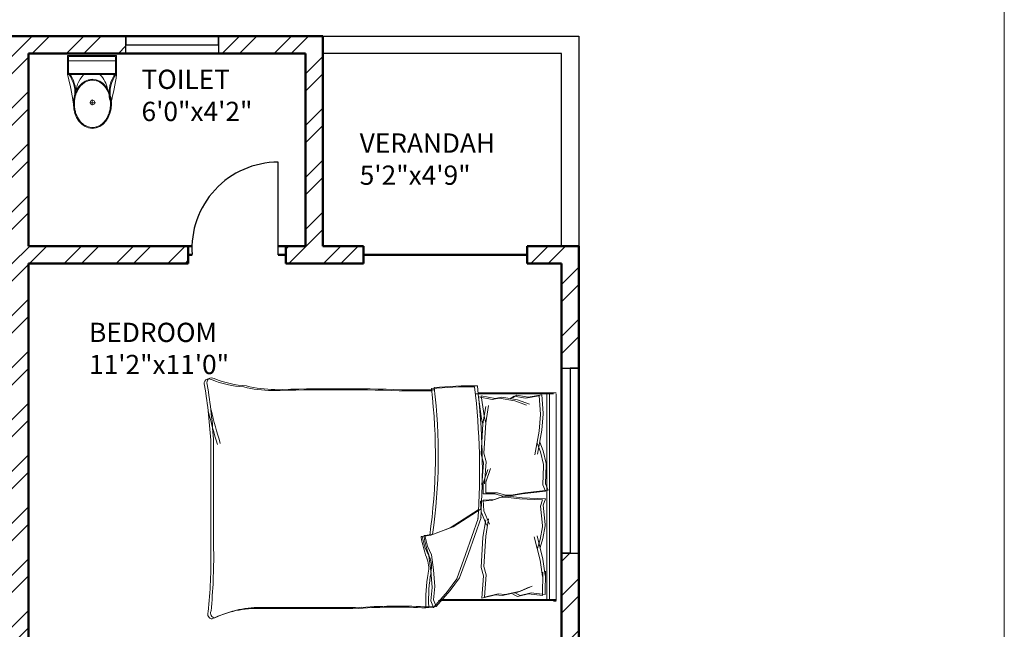
# Model space of a CAD drawing. Units: inches. Extents: x 1901 to 2863, y 888 to 2433.
# Tile 91 of 91: x 2608 to 2863, y 2120 to 2278. Entities that reach past the tile are written whole.
import ezdxf

# ---------------------------------------------------------------- set-up
doc = ezdxf.new("R2010")
doc.units = ezdxf.units.IN
for name, color, linetype, lineweight in [('A-AREA-IDEN', 7, 'Continuous', 18), ('A-DOOR', 4, 'Continuous', 25), ('A-FLOR-FIXT', 9, 'Continuous', 18), ('A-FLOR-HRAL', 41, 'Continuous', 25), ('A-FURN', 8, 'Continuous', 18), ('A-GLAZ', 3, 'Continuous', 25), ('A-WALL', 7, 'Continuous', 50), ('A-WALL-PATT', 8, 'Continuous', 13)]:
    doc.layers.add(name, color=color, linetype=linetype, lineweight=lineweight)
doc.styles.get("Standard").update_dxf_attribs({"font": 'arial.ttf'})

# ---------------------------------------------------------------- blocks, each defined once
blk = doc.blocks.new('A$C31115884')
for p, q in [((258, 466), (258, 523)), ((283, 498), (223, 498)), ((0, 200), (0, 0)), ((520, 200), (0, 200)), ((10, 190), (10, 10)), ((510, 190), (10, 190)), ((510, 10), (510, 190)), ((520, 0), (520, 200)), ((510, 54), (0, 54)), ((10, 10), (510, 10)), ((0, 0), (520, 0))]:
    blk.add_line(p, q)
blk.add_circle((256, 496), 23.6)
for centre, radius, start, end in [((2778, -205), 2807, 165.4549, 171.7133), ((-295, 403), 365, 324.2091, 9.3499), ((-295, 403), 375, 324.2091, 9.3499), ((139, 406), 293, 315.8436, 2.6563), ((806, 403), 365, 170.6501, 215.7909), ((3237, 905), 2807, 188.2867, 194.5451), ((384, 406), 293, 190.2774, 224.1564), ((806, 403), 375, 179.2036, 215.7909)]:
    blk.add_arc(centre, radius, start, end)
blk.add_ellipse((256, 510), major_axis=(0, -261), ratio=0.772727)
blk.add_open_spline([(256, 259), (263, 259), (270, 260), (288, 262), (299, 265), (320, 273), (330, 278), (350, 291), (360, 299), (378, 316), (386, 326), (402, 347), (409, 358), (421, 383), (427, 395), (436, 422), (440, 436), (445, 465), (447, 480), (448, 509), (448, 524), (445, 553), (443, 568), (436, 596), (432, 610), (422, 636), (416, 649), (402, 672), (395, 683), (379, 703), (370, 712), (351, 728), (341, 735), (321, 746), (310, 751), (289, 757), (278, 759), (256, 761), (245, 761), (223, 757), (212, 754), (191, 746), (181, 741), (161, 728), (151, 720), (133, 703), (125, 693), (110, 672), (103, 660), (90, 636), (85, 623), (76, 596), (72, 582), (67, 553), (66, 538), (64, 509), (65, 494), (68, 465), (70, 450), (77, 422), (81, 408), (91, 382), (97, 370), (111, 346), (118, 335), (135, 316), (144, 307), (162, 291), (172, 284), (193, 273), (203, 269), (225, 262), (236, 260), (250, 259), (253, 259), (256, 259)], degree=3, knots=[0, 0, 0, 0, 0.110105, 0.110105, 0.285049, 0.285049, 0.459994, 0.459994, 0.634938, 0.634938, 0.809882, 0.809882, 0.984827, 0.984827, 1.159771, 1.159771, 1.334715, 1.334715, 1.50966, 1.50966, 1.684604, 1.684604, 1.859549, 1.859549, 2.034493, 2.034493, 2.209437, 2.209437, 2.384382, 2.384382, 2.559326, 2.559326, 2.73427, 2.73427, 2.909215, 2.909215, 3.084159, 3.084159, 3.259103, 3.259103, 3.434048, 3.434048, 3.608992, 3.608992, 3.783936, 3.783936, 3.958881, 3.958881, 4.133825, 4.133825, 4.30877, 4.30877, 4.483714, 4.483714, 4.658658, 4.658658, 4.833603, 4.833603, 5.008547, 5.008547, 5.183491, 5.183491, 5.358436, 5.358436, 5.53338, 5.53338, 5.708324, 5.708324, 5.883269, 5.883269, 6.058213, 6.058213, 6.233158, 6.233158, 6.283185, 6.283185, 6.283185, 6.283185])
blk = doc.blocks.new('BED-DOUBLE')
for p, q in [((31.18, 59.32), (27.53, 55.16)), ((31.18, 59.32), (27.53, 55.16)), ((31.9, 59.58), (28.25, 55.42)), ((31.9, 59.58), (28.25, 55.42)), ((33.14, 59.41), (31.18, 59.32, 4.35)), ((33.14, 59.41), (31.18, 59.32, 4.35)), ((31.87, 57.59), (31.18, 59.32)), ((31.87, 57.59), (31.18, 59.32)), ((33.85, 59.67), (31.9, 59.58, 4.35)), ((33.85, 59.67), (31.9, 59.58, 4.35)), ((32.59, 57.85), (31.9, 59.58)), ((32.59, 57.85), (31.9, 59.58)), ((0.03, 57.78), (0.03, 4.12)), ((0.74, 57.78), (30.62, 57.78)), ((0.74, 57.78), (30.62, 57.78)), ((3.61, 56.48), (3.51, 50.42)), ((3.61, 56.48), (3.51, 50.42)), ((3.61, 56.48), (7.22, 56.06)), ((3.61, 56.48), (7.22, 56.06)), ((6.5, 55.8), (9.39, 56.47)), ((6.5, 55.8), (9.39, 56.47)), ((7.22, 56.06), (10.11, 56.73)), ((7.22, 56.06), (10.11, 56.73)), ((9.39, 56.47), (10.56, 55.89)), ((9.39, 56.47), (10.56, 55.89)), ((14.02, 56.48), (10.01, 55.58)), ((14.02, 56.48), (10.01, 55.58)), ((10.11, 56.73), (11.28, 56.15)), ((10.11, 56.73), (11.28, 56.15)), ((15.83, 56.27), (14.02, 56.48)), ((15.83, 56.27), (14.02, 56.48)), ((18.63, 56.89), (15.11, 56.01)), ((18.63, 56.88), (15.11, 56.01)), ((19.35, 57.14), (15.83, 56.27)), ((19.35, 57.14), (15.83, 56.27)), ((18.18, 51.12), (18.63, 56.89)), ((18.18, 51.12), (18.63, 56.88)), ((18.9, 51.38), (19.35, 57.14)), ((18.9, 51.38), (19.35, 57.14)), ((31.53, 54.12), (31.87, 57.59)), ((31.53, 54.12), (31.87, 57.59)), ((32.24, 54.37), (32.59, 57.85)), ((32.24, 54.37), (32.59, 57.85)), ((2.9, 56.23), (2.79, 50.16)), ((2.9, 56.23), (2.79, 50.16)), ((2.9, 56.23), (6.5, 55.8)), ((2.9, 56.23), (6.5, 55.8)), ((9.3, 55.33), (6.29, 54)), ((9.3, 55.33), (6.29, 54)), ((10.01, 55.58), (7.01, 54.26)), ((10.01, 55.58), (7.01, 54.26)), ((13.31, 56.23), (9.3, 55.33)), ((13.31, 56.23), (9.3, 55.33)), ((15.11, 56.01), (13.31, 56.23)), ((15.11, 56.01), (13.31, 56.23)), ((27.53, 55.16), (25.1, 51.86)), ((27.53, 55.16), (25.1, 51.86)), ((28.25, 55.42), (25.81, 52.11)), ((28.25, 55.42), (25.81, 52.11)), ((31.87, 49.77), (31.53, 54.12)), ((31.87, 49.77), (31.53, 54.12)), ((32.59, 50.03), (32.24, 54.37)), ((32.59, 50.03), (32.24, 54.37)), ((2.79, 50.16), (2.88, 51.29)), ((2.79, 50.16), (2.88, 51.29)), ((2.88, 51.29), (3.47, 47.02)), ((2.88, 51.29), (3.47, 47.02)), ((3.51, 50.42), (3.6, 51.54)), ((3.51, 50.42), (3.6, 51.54)), ((3.6, 51.54), (4.19, 47.28)), ((3.6, 51.54), (4.19, 47.28)), ((19.52, 49.18), (18.9, 51.38)), ((19.52, 49.18), (18.9, 51.38)), ((25.1, 51.86), (22.84, 45.6)), ((25.1, 51.86), (22.84, 45.6)), ((25.81, 52.11), (23.55, 45.85)), ((25.81, 52.11), (23.55, 45.85)), ((18.81, 48.92), (18.18, 51.12)), ((18.81, 48.92), (18.18, 51.12)), ((18.32, 41.05), (18.81, 48.92)), ((18.32, 41.05), (18.81, 48.92)), ((19.04, 41.31), (19.52, 49.18)), ((19.04, 41.31), (19.52, 49.18)), ((32.39, 45.94), (31.87, 49.77)), ((32.39, 45.94), (31.87, 49.77)), ((33.11, 46.2), (32.59, 50.03)), ((33.11, 46.2), (32.59, 50.03)), ((3.47, 47.02), (4.99, 40.94)), ((3.47, 47.02), (4.99, 40.94)), ((4.19, 47.28), (5.71, 41.19)), ((4.19, 47.28), (5.71, 41.19)), ((34.15, 43.94), (33.11, 46.2)), ((34.15, 43.94), (33.11, 46.2)), ((4.15, 43.98), (3.48, 41.66)), ((4.15, 43.98), (3.48, 41.66)), ((4.87, 44.23), (4.2, 41.91)), ((4.87, 44.23), (4.2, 41.91)), ((22.84, 45.6), (19.54, 36.24)), ((22.84, 45.6), (19.54, 36.24)), ((23.55, 45.85), (20.26, 36.49)), ((23.55, 45.85), (20.26, 36.49)), ((33.44, 43.68), (32.39, 45.94)), ((33.44, 43.68), (32.39, 45.94)), ((34.13, 40.9), (33.44, 43.68)), ((34.13, 40.9), (33.44, 43.68)), ((34.85, 41.16), (34.15, 43.94)), ((34.85, 41.16), (34.15, 43.94)), ((89, 16.88), (89, 44.51)), ((89, 16.88), (89, 44.51)), ((89.72, 17.13), (89.72, 44.77)), ((89.72, 17.13), (89.72, 44.77)), ((3.48, 41.66), (2.87, 38.37)), ((3.48, 41.66), (2.87, 38.37)), ((4.2, 41.91), (3.59, 38.62)), ((4.2, 41.91), (3.59, 38.62)), ((17.57, 36.53), (18.32, 41.05)), ((17.57, 36.52), (18.32, 41.05)), ((18.29, 36.78), (19.04, 41.31)), ((18.29, 36.78), (19.04, 41.31)), ((32.59, 40.81), (34.85, 41.16)), ((32.59, 40.81), (34.85, 41.16)), ((2.87, 38.37), (2.9, 38.01)), ((2.87, 38.37), (2.9, 38.01)), ((3.59, 38.62), (3.62, 38.26)), ((3.59, 38.62), (3.62, 38.26)), ((19.54, 33.94), (26.83, 38.64)), ((19.54, 33.94), (26.83, 38.64)), ((20.26, 34.19), (27.55, 38.9)), ((20.26, 34.19), (27.55, 38.9)), ((26.83, 38.64), (31.87, 40.55)), ((26.83, 38.64), (31.87, 40.55)), ((27.55, 38.9), (32.59, 40.81)), ((27.55, 38.9), (32.59, 40.81)), ((31.87, 40.55), (34.13, 40.9)), ((31.87, 40.55), (34.13, 40.9)), ((2.9, 38.01), (3.37, 33.03)), ((2.9, 38.01), (3.37, 33.04)), ((3.62, 38.26), (4.09, 33.29)), ((3.62, 38.26), (4.09, 33.29)), ((18.82, 34.49), (17.38, 37.94)), ((18.82, 34.49), (17.38, 37.94)), ((19.54, 34.74), (18.1, 38.19)), ((19.54, 34.74), (18.1, 38.19)), ((4.09, 33.29), (3.54, 31.63)), ((4.09, 33.29), (3.54, 31.63)), ((18.99, 31.73), (18.82, 34.49)), ((18.99, 31.73), (18.82, 34.49)), ((19.71, 31.99), (19.54, 34.74)), ((19.71, 31.99), (19.54, 34.74)), ((3.37, 33.04), (2.82, 31.37)), ((3.37, 33.03), (2.82, 31.37)), ((2.82, 31.37), (8.86, 31.1)), ((2.82, 31.37), (8.86, 31.1)), ((3.54, 31.63), (9.58, 31.36)), ((3.54, 31.63), (9.58, 31.36)), ((8.86, 31.1), (12.46, 30.68)), ((8.86, 31.1), (12.46, 30.68)), ((9.58, 31.36), (13.18, 30.93)), ((9.58, 31.36), (13.18, 30.93)), ((12.46, 30.68), (13.92, 30.77)), ((12.46, 30.68), (13.92, 30.77)), ((13.18, 30.93), (14.64, 31.02)), ((13.18, 30.93), (14.64, 31.02)), ((13.92, 30.77), (15.99, 31.55)), ((13.92, 30.77), (15.99, 31.55)), ((14.64, 31.02), (16.71, 31.8)), ((14.64, 31.02), (16.71, 31.8)), ((15.99, 31.55), (18.99, 31.73)), ((15.99, 31.55), (18.99, 31.73)), ((16.71, 31.8), (19.71, 31.99)), ((16.71, 31.8), (19.71, 31.99)), ((2.13, 29.14), (8.13, 29.78)), ((2.13, 29.14), (8.13, 29.78)), ((2.78, 27.51), (2.13, 29.14)), ((2.78, 27.51), (2.13, 29.14)), ((2.84, 29.39), (8.85, 30.04)), ((2.84, 29.39), (8.85, 30.04)), ((3.49, 27.77), (2.84, 29.39)), ((3.49, 27.77), (2.84, 29.39)), ((8.13, 29.78), (11.7, 30.43)), ((8.13, 29.78), (11.7, 30.43)), ((8.85, 30.04), (12.42, 30.69)), ((8.85, 30.04), (12.42, 30.69)), ((11.7, 30.43), (13.16, 30.43)), ((11.7, 30.43), (13.16, 30.43)), ((12.42, 30.69), (13.88, 30.69)), ((12.42, 30.69), (13.88, 30.69)), ((13.16, 30.43), (15.28, 29.78)), ((13.16, 30.43), (15.28, 29.78)), ((13.88, 30.69), (15.99, 30.04)), ((13.88, 30.69), (15.99, 30.04)), ((15.28, 29.78), (18.29, 29.78)), ((15.28, 29.78), (18.29, 29.78)), ((15.99, 30.04), (19, 30.04)), ((15.99, 30.04), (19, 30.04)), ((18.29, 29.78), (18.29, 27.03)), ((18.29, 29.78), (18.29, 27.03)), ((19, 30.04), (19, 27.28)), ((19, 30.04), (19, 27.28)), ((2.61, 22.52), (2.78, 27.51)), ((2.61, 22.52), (2.78, 27.51)), ((3.33, 22.78), (3.49, 27.77)), ((3.33, 22.78), (3.49, 27.77)), ((18.29, 27.03), (17.06, 23.49)), ((18.29, 27.03), (17.06, 23.5)), ((19, 27.28), (17.78, 23.75)), ((19, 27.28), (17.78, 23.75)), ((18.18, 21.73), (18.63, 27.49)), ((18.18, 21.73), (18.63, 27.49)), ((18.9, 21.98), (19.35, 27.75)), ((18.9, 21.98), (19.35, 27.74)), ((2.61, 22.16), (2.61, 22.52)), ((2.61, 22.16), (2.61, 22.52)), ((3.42, 18.91), (2.61, 22.16)), ((3.42, 18.91), (2.61, 22.16)), ((3.33, 22.42), (3.33, 22.78)), ((3.33, 22.42), (3.33, 22.78)), ((4.14, 19.17), (3.33, 22.42)), ((4.14, 19.17), (3.33, 22.42)), ((18.81, 19.53), (18.18, 21.73)), ((18.81, 19.53), (18.18, 21.73)), ((19.52, 19.78), (18.9, 21.98)), ((19.52, 19.78), (18.9, 21.98)), ((4.24, 16.64), (3.42, 18.91)), ((4.24, 16.64), (3.42, 18.91)), ((3.75, 13.56), (4.89, 19.73)), ((3.75, 13.56), (4.89, 19.73)), ((4.95, 16.9), (4.14, 19.17)), ((4.95, 16.9), (4.14, 19.17)), ((4.47, 13.81), (5.6, 19.98)), ((4.47, 13.81), (5.6, 19.98)), ((18.32, 11.66), (18.81, 19.53)), ((18.32, 11.66), (18.81, 19.53)), ((19.04, 11.91), (19.52, 19.78)), ((19.04, 11.91), (19.52, 19.78)), ((3.42, 9.27), (3.75, 13.56)), ((3.42, 9.27), (3.75, 13.56)), ((4.14, 9.52), (4.47, 13.81)), ((4.14, 9.52), (4.47, 13.81)), ((17.57, 7.13), (18.32, 11.66)), ((17.57, 7.13), (18.32, 11.66)), ((18.29, 7.38), (19.04, 11.91)), ((18.29, 7.39), (19.04, 11.91)), ((18.32, 11.66), (18.68, 10.38)), ((18.32, 11.66), (18.68, 10.38)), ((18.68, 10.38), (19.5, 4.66)), ((18.68, 10.38), (19.5, 4.66)), ((19.04, 11.91), (19.4, 10.64)), ((19.04, 11.91), (19.4, 10.64)), ((19.4, 10.64), (20.21, 4.92)), ((19.4, 10.64), (20.21, 4.92)), ((3.4, 9.15), (3.42, 9.27)), ((3.4, 9.15), (3.42, 9.27)), ((3.77, 4.34), (3.4, 9.15)), ((3.77, 4.34), (3.4, 9.15)), ((4.12, 9.4), (4.14, 9.52)), ((4.12, 9.4), (4.14, 9.52)), ((4.49, 4.6), (4.12, 9.4)), ((4.49, 4.6), (4.12, 9.4)), ((4.47, 4.59), (8.04, 5.24)), ((4.47, 4.59), (8.04, 5.24)), ((10.08, 5.63), (7, 6.77)), ((10.08, 5.63), (7, 6.77)), ((10.8, 5.89), (7.71, 7.03)), ((10.8, 5.89), (7.71, 7.03)), ((8.04, 5.24), (10.96, 4.75)), ((8.04, 5.24), (10.96, 4.76)), ((14.14, 4.99), (10.08, 5.63)), ((14.14, 4.99), (10.08, 5.63)), ((10.24, 4.5), (11.38, 5.15)), ((10.24, 4.5), (11.38, 5.15)), ((14.86, 5.24), (10.8, 5.89)), ((14.86, 5.24), (10.8, 5.89)), ((10.96, 4.76), (12.1, 5.4)), ((10.96, 4.75), (12.1, 5.4)), ((15.92, 5.31), (14.14, 4.99)), ((15.92, 5.31), (14.14, 4.99)), ((16.64, 5.57), (14.86, 5.24)), ((16.64, 5.57), (14.86, 5.24)), ((19.5, 4.66), (15.92, 5.31)), ((19.5, 4.66), (15.92, 5.31)), ((20.21, 4.92), (16.64, 5.57)), ((20.21, 4.92), (16.64, 5.57)), ((3.75, 4.34), (7.32, 4.99)), ((3.75, 4.34), (7.32, 4.99)), ((7.32, 4.99), (10.24, 4.5)), ((7.32, 4.99), (10.24, 4.5))]:
    blk.add_line(p, q)
for centre, radius, start, end in [((77.12, 85.47), 25.9, 267.4714, 296.4681), ((77.12, 85.47), 25.9, 267.4714, 296.4681), ((77.84, 85.73), 25.9, 267.4714, 296.4681), ((77.84, 85.73), 25.9, 267.4714, 296.4681), ((88.58, 61.05), 1.24, 332.6588, 86.02), ((88.58, 61.05), 1.24, 332.6588, 86.02), ((89.3, 61.31), 1.24, 332.6588, 86.02), ((89.3, 61.31), 1.24, 332.6588, 86.02), ((-7.45, 57.59), 40.62, 349.8763, 2.5657), ((-7.45, 57.59), 40.62, 349.8763, 2.5657), ((40.8, 204.6), 145.39, 266.9791, 273.8365), ((40.8, 204.6), 145.39, 266.9791, 273.8365), ((-6.73, 57.85), 40.62, 349.8763, 2.5657), ((-6.73, 57.85), 40.62, 349.8763, 2.5657), ((41.52, 204.86), 145.39, 266.9791, 273.8365), ((41.52, 204.86), 145.39, 266.9791, 273.8365), ((76.17, -5062.23), 5121.82, 90.00217, 90.28689), ((76.17, -5062.23), 5121.82, 90.00217, 90.28689), ((76.89, -5061.97), 5121.82, 90.00217, 90.28689), ((76.89, -5061.97), 5121.82, 90.00217, 90.28689), ((238.36, 46.17), 149.37, 174.4998, 180.6351), ((238.36, 46.17), 149.37, 174.4998, 180.6351), ((239.08, 46.42), 149.37, 174.4998, 180.6351), ((239.08, 46.42), 149.37, 174.4998, 180.6351), ((39.4, 49.08), 6.99, 168.6608, 203.7384), ((39.4, 49.08), 6.99, 168.6608, 203.7384), ((40.11, 49.33), 6.99, 168.6608, 203.7384), ((40.11, 49.33), 6.99, 168.6608, 203.7384), ((1.69, 34.94), 33.29, 10.6617, 19.8806), ((1.69, 34.94), 33.29, 10.6617, 19.8806), ((2.41, 35.2), 33.29, 10.6617, 19.8806), ((2.41, 35.2), 33.29, 10.6617, 19.8806), ((34.2, 41.1), 0.207, 250.2464, 1.1377), ((34.2, 41.1), 0.207, 250.2464, 1.1377), ((34.92, 41.35), 0.207, 250.2464, 1.1377), ((34.92, 41.35), 0.207, 250.2464, 1.1377), ((175.53, 19.9), 144.86, 171.7845, 186.9006), ((175.53, 19.9), 144.86, 171.7845, 186.9006), ((176.25, 20.16), 144.86, 171.7845, 186.9006), ((176.25, 20.15), 144.86, 171.7845, 186.9006), ((204.43, 23.94), 185.22, 176.0865, 186.7821), ((204.43, 23.94), 185.22, 176.0865, 186.7821), ((205.14, 24.2), 185.22, 176.0865, 186.7821), ((205.14, 24.2), 185.22, 176.0865, 186.7821), ((225.52, 24.02), 136.7, 182.9958, 189.4091), ((225.52, 24.02), 136.7, 182.9958, 189.4091), ((226.23, 24.28), 136.7, 182.9958, 189.4091), ((226.23, 24.28), 136.7, 182.9958, 189.4091), ((23.31, 95.84), 93.53, 268.7218, 275.604), ((23.31, 95.84), 93.53, 268.7218, 275.604), ((35.03, -187.88), 190.99, 88.4762, 91.0082), ((35.03, -187.88), 190.99, 88.4762, 91.0082), ((35.74, -187.62), 190.99, 88.4762, 91.0082), ((35.74, -187.62), 190.99, 88.4762, 91.0082), ((56.85, 544.3), 541.51, 268.2277, 271.7185), ((56.85, 544.3), 541.51, 268.2277, 271.7185), ((57.57, 544.55), 541.51, 268.2277, 271.7185), ((57.57, 544.55), 541.51, 268.2277, 271.7185), ((72.46, -30.24), 33.27, 76.0648, 88.9113), ((72.46, -30.24), 33.27, 76.0648, 88.9113), ((73.18, -29.98), 33.27, 76.0648, 88.9113), ((73.18, -29.98), 33.27, 76.0648, 88.9113), ((22.59, 95.58), 93.53, 268.7218, 275.604), ((22.59, 95.58), 93.53, 268.7218, 275.604), ((78.93, -24.35), 26.45, 67.9751, 86.652), ((78.93, -24.35), 26.45, 67.9751, 86.652), ((79.65, -24.1), 26.45, 67.9751, 86.652), ((79.65, -24.1), 26.45, 67.9751, 86.652), ((89.53, 1.18), 1.22, 236.1736, 23.4781), ((89.53, 1.18), 1.22, 236.1736, 23.4781), ((90.25, 1.44), 1.22, 236.1736, 23.4781), ((90.25, 1.44), 1.22, 236.1736, 23.4781)]:
    blk.add_arc(centre, radius, start, end)
blk = doc.blocks.new('WIN-48')
for p, q in [((0, 2.25), (0, 4.5)), ((0, 4.5), (0, 0)), ((48, 4.5), (48, 0)), ((48, 2.25), (0, 2.25)), ((48, 0), (48, 2.25))]:
    blk.add_line(p, q)
blk = doc.blocks.new('WIN-24-3')
for p, q in [((0, 0), (0, 4.5)), ((0, 4.5), (0, 2.25)), ((24, 2.25), (24, 4.5)), ((24, 4.5), (24, 0)), ((0, 2.25), (24, 2.25))]:
    blk.add_line(p, q)

msp = doc.modelspace()

# ---------------------------------------------------------------- hatches: boundary and pattern name
at = {"layer": 'A-WALL-PATT'}
h = msp.add_hatch(dxfattribs=at)
h.set_pattern_fill('ANSI32', color=256)
h.paths.add_polyline_path([(2192.5, 2274.13), (2141.26, 2274.13), (2141.26, 2269.63), (2192.5, 2269.63)])
h.paths.add_polyline_path([(2259.93, 2274.13), (2216.5, 2274.13), (2216.5, 2269.63), (2255.43, 2269.63), (2255.43, 2214.63), (2250.81, 2214.63), (2250.81, 2210.13), (2259.93, 2210.13), (2259.93, 2215.13), (2271.76, 2215.13), (2271.76, 2217.38), (2271.76, 2219.63), (2259.93, 2219.63)])
h.paths.add_polyline_path([(2171.43, 2269.63), (2166.93, 2269.63), (2166.93, 2219.63), (2121.24, 2219.63), (2121.24, 2215.13), (2166.93, 2215.13), (2166.93, 2083.13), (2161.81, 2083.13), (2161.81, 2078.63), (2171.43, 2078.63), (2177, 2078.63), (2177, 2080.88), (2177, 2083.13), (2171.43, 2083.13), (2171.43, 2210.13), (2230.91, 2210.13), (2230.91, 2212.38), (2230.91, 2214.63), (2171.43, 2214.63)])
h.paths.add_polyline_path([(2117.26, 2274.13), (2089.43, 2274.13), (2089.43, 2219.63), (2081.14, 2219.63), (2081.14, 2215.13), (2089.43, 2215.13), (2098, 2215.13), (2098, 2217.38), (2098, 2219.63), (2093.93, 2219.63), (2093.93, 2269.63), (2117.26, 2269.63), (2117.26, 2271.88)])
h.paths.add_polyline_path([(2343.43, 2219.63), (2329.29, 2219.63), (2329.29, 2215.13), (2338.93, 2215.13), (2338.93, 2184.74), (2343.43, 2184.74)])
h.paths.add_polyline_path([(2338.93, 2083.13), (2329.29, 2083.13), (2208.97, 2083.13), (2208.97, 2078.63), (2338.93, 2078.63)])
h.paths.add_polyline_path([(2343.43, 2136.74), (2338.93, 2136.74), (2338.93, 1872.63), (2343.43, 1872.63)])
h.paths.add_polyline_path([(2343.43, 1863.63), (2397.68, 1863.63), (2397.68, 1821.63), (2384.14, 1821.63), (2384.14, 1812.63), (2418.33, 1812.63), (2418.33, 1817.13), (2418.33, 1821.63), (2406.68, 1821.63), (2406.68, 1863.63), (2459.5, 1863.63), (2459.5, 1821.63), (2447.14, 1821.63), (2447.14, 1812.63), (2459.5, 1812.63), (2468.5, 1812.63), (2468.5, 1872.63), (2394.43, 1872.63), (2334.43, 1872.63), (2334.43, 1812.63), (2343.43, 1812.63), (2353.25, 1812.63), (2353.25, 1821.63), (2343.43, 1821.63)])
h.paths.add_polyline_path([(2510.01, 1872.63), (2468.5, 1872.63), (2468.5, 1868.13), (2510.01, 1868.13)])
h.paths.add_polyline_path([(2514.01, 1817.13), (2468.5, 1817.13), (2468.5, 1812.63), (2482.11, 1812.63), (2482.11, 1800.61), (2486.61, 1800.61), (2486.61, 1812.63), (2514.01, 1812.63)])
h.paths.add_polyline_path([(2299.25, 1814.88), (2299.25, 1817.13), (2295.93, 1817.13), (2295.93, 1854.17), (2293.68, 1854.17), (2291.43, 1854.17), (2291.43, 1817.13), (2266.11, 1817.13), (2266.11, 1812.63), (2299.25, 1812.63)])
h.paths.add_polyline_path([(2218.11, 1817.13), (2206.46, 1817.13), (2171.43, 1817.13), (2171.43, 1949.13), (2190.1, 1949.13), (2190.1, 1953.63), (2163.47, 1953.63), (2163.47, 1949.13), (2166.93, 1949.13), (2166.93, 1817.13), (2114.3, 1817.13), (2114.3, 1812.63), (2218.11, 1812.63)])
h.paths.add_polyline_path([(2029.43, 1970.92), (2024.93, 1970.92), (2024.93, 1912.72), (2029.43, 1912.72)])
h.paths.add_polyline_path([(2132.3, 1953.63), (2113.93, 1953.63), (2113.93, 1975.89), (2111.68, 1975.89), (2109.43, 1975.89), (2109.43, 1953.63), (2029.43, 1953.63), (2029.43, 1949.13), (2132.3, 1949.13)])
h.paths.add_polyline_path([(2029.43, 1853.61), (2029.31, 1853.61), (2029.31, 1853.61), (2029.43, 1853.61), (2029.43, 1864.72), (2024.93, 1864.72), (2024.93, 1812.63), (2066.3, 1812.63), (2066.3, 1814.88), (2066.3, 1817.13), (2029.43, 1817.13)])
h.paths.add_polyline_path([(2122.93, 2010.09), (2120.68, 2010.09), (2118.43, 2010.09), (2118.43, 2006.13), (2029.43, 2006.13), (2029.43, 2001.63), (2109.43, 2001.63), (2109.43, 1998.04), (2113.93, 1998.04), (2113.93, 2001.63), (2122.93, 2001.63)])
h.paths.add_polyline_path([(2029.43, 2031.38), (2024.93, 2031.38), (2024.93, 1994.92), (2027.18, 1994.92), (2029.43, 1994.92)])
h.paths.add_polyline_path([(2029.43, 2136.74), (2024.93, 2136.74), (2024.93, 2067.38), (2027.18, 2067.38), (2029.43, 2067.38)])
h.paths.add_polyline_path([(2125.62, 2083.13), (2029.43, 2083.13), (2029.43, 2078.63), (2118.43, 2078.63), (2118.43, 2030.71), (2122.93, 2030.71), (2122.93, 2078.63), (2125.62, 2078.63)])
h.paths.add_polyline_path([(2029.43, 2215.13), (2040.47, 2215.13), (2040.47, 2217.38), (2040.47, 2219.63), (2024.93, 2219.63), (2024.93, 2184.74), (2029.43, 2184.74), (2029.43, 2187.78)])
h.paths.add_polyline_path([(2686.43, 2274.13), (2659.28, 2274.13), (2659.28, 2269.63), (2681.93, 2269.63), (2681.93, 2219.63), (2676.82, 2219.63), (2676.82, 2215.13), (2681.93, 2215.13), (2697.01, 2215.13), (2697.01, 2217.38), (2697.01, 2219.63), (2686.43, 2219.63)])
h.paths.add_polyline_path([(2609.93, 2269.63), (2635.28, 2269.63), (2635.28, 2274.13), (2571.43, 2274.13), (2571.43, 2269.63), (2605.43, 2269.63), (2605.43, 2214.63), (2549.1, 2214.63), (2549.1, 2210.13), (2605.43, 2210.13), (2605.43, 2083.13), (2601.01, 2083.13), (2601.01, 2080.88), (2601.01, 2078.63), (2609.93, 2078.63), (2616.16, 2078.63), (2616.16, 2080.88), (2616.16, 2083.13), (2609.93, 2083.13), (2609.93, 2215.13), (2651.46, 2215.13), (2651.46, 2217.38), (2651.46, 2219.63), (2609.93, 2219.63)])
h.paths.add_polyline_path([(2521.43, 2269.63), (2547.43, 2269.63), (2547.43, 2271.88), (2547.43, 2274.13), (2516.93, 2274.13), (2516.93, 2219.63), (2506.41, 2219.63), (2506.41, 2215.13), (2516.93, 2215.13), (2516.93, 2210.13), (2525.4, 2210.13), (2525.4, 2212.38), (2525.4, 2214.63), (2521.43, 2214.63)])
h.paths.add_polyline_path([(2456.01, 2219.63), (2439.43, 2219.63), (2439.43, 2187.89), (2443.93, 2187.89), (2443.93, 2215.13), (2456.01, 2215.13)])
h.paths.add_polyline_path([(2752.93, 2219.63), (2739.48, 2219.63), (2739.48, 2215.13), (2748.43, 2215.13), (2748.43, 2187.89), (2752.93, 2187.89)])
h.paths.add_polyline_path([(2752.93, 2139.89), (2748.43, 2139.89), (2748.43, 2083.13), (2648.42, 2083.13), (2648.42, 2078.63), (2654.93, 2078.63), (2654.93, 2039.44), (2659.43, 2039.44), (2659.43, 2078.63), (2748.43, 2078.63), (2748.43, 2063.43), (2752.93, 2063.43)])
h.paths.add_polyline_path([(2752.93, 2010.63), (2659.43, 2010.63), (2659.43, 2015.65), (2654.93, 2015.65), (2654.93, 2010.63), (2605.43, 2010.63), (2605.43, 1920.97), (2609.93, 1920.97), (2609.93, 2006.13), (2748.43, 2006.13), (2748.43, 1982.47), (2752.93, 1982.47)])
h.paths.add_polyline_path([(2752.93, 2027.43), (2748.43, 2027.43), (2748.43, 2010.63), (2752.93, 2010.63)])
h.paths.add_polyline_path([(2748.43, 1886.13), (2609.93, 1886.13), (2609.93, 1889.72), (2605.43, 1889.72), (2605.43, 1861.26), (2609.93, 1861.26), (2609.93, 1881.63), (2748.43, 1881.63)])
h.paths.add_polyline_path([(2456.86, 2228.83), (2498.4, 2228.83), (2498.4, 2247.49), (2456.86, 2247.49)], flags=9)
h.paths.add_polyline_path([(2038.6, 2237.42), (2080.17, 2237.42), (2080.17, 2256.08), (2038.6, 2256.08)], flags=9)
h.paths.add_polyline_path([(2292.01, 1062.39), (2539.93, 1062.39), (2539.93, 1099.49), (2292.01, 1099.49)], flags=9)
h.paths.add_polyline_path([(2424.91, 1832.25), (2448.51, 1832.25), (2448.51, 1846.68), (2424.91, 1846.68)], flags=25)
h.paths.add_polyline_path([(2359.08, 1832.25), (2382.68, 1832.25), (2382.68, 1846.68), (2359.08, 1846.68)], flags=25)
h.paths.add_polyline_path([(2352.9, 1684.8), (2367.54, 1684.8), (2367.54, 1697.17), (2352.9, 1697.17)], flags=9)
h.paths.add_polyline_path([(2079.29, 1755.83), (2169.02, 1755.83), (2169.02, 1774.37), (2079.29, 1774.37)], flags=9)
h.paths.add_polyline_path([(2404.09, 1373.86), (2404.09, 1463.59), (2385.54, 1463.59), (2385.54, 1373.86)], flags=9)
h.paths.add_polyline_path([(2268.09, 2236.37), (2309.64, 2236.37), (2309.64, 2255.03), (2268.09, 2255.03)], flags=9)
h.paths.add_polyline_path([(2575.96, 1700.95), (2665.7, 1700.95), (2665.7, 1719.5), (2575.96, 1719.5)], flags=9)
h.paths.add_polyline_path([(2302.96, 1878.47), (2329.52, 1878.47), (2329.52, 1888.78), (2302.96, 1888.78)], flags=9)
h.paths.add_polyline_path([(2097.42, 2240.58), (2126.57, 2240.58), (2126.57, 2259.23), (2097.42, 2259.23)], flags=9)
h.paths.add_polyline_path([(2208.72, 2246.12), (2237.88, 2246.12), (2237.88, 2264.78), (2208.72, 2264.78)], flags=9)
h.paths.add_polyline_path([(2038.15, 1925.96), (2076.99, 1925.96), (2076.99, 1944.62), (2038.15, 1944.62)], flags=9)
h.paths.add_polyline_path([(2239.14, 1926.67), (2288.46, 1926.67), (2288.46, 1945.33), (2239.14, 1945.33)], flags=9)
h.paths.add_polyline_path([(2175.43, 2007.33), (2212.36, 2007.33), (2212.36, 2025.99), (2175.43, 2025.99)], flags=9)
h.paths.add_polyline_path([(2225.03, 2091.79), (2263.87, 2091.79), (2263.87, 2110.45), (2225.03, 2110.45)], flags=9)
h.paths.add_polyline_path([(2035.4, 2098.48), (2074.24, 2098.48), (2074.24, 2117.14), (2035.4, 2117.14)], flags=9)
h.paths.add_polyline_path([(2050.1, 2029.21), (2083.26, 2029.21), (2083.26, 2047.87), (2050.1, 2047.87)], flags=9)
h.paths.add_polyline_path([(2069.68, 1956.72), (2098.83, 1956.72), (2098.83, 1975.38), (2069.68, 1975.38)], flags=25)
h.paths.add_polyline_path([(2328.62, 1753.34), (2361.66, 1753.34), (2361.66, 1771.99), (2328.62, 1771.99)], flags=9)
h.paths.add_polyline_path([(2395.16, 2060.89), (2395.16, 2140.65), (2378.68, 2140.65), (2378.68, 2060.89)], flags=9)
h.paths.add_polyline_path([(2463.73, 2059.02), (2492.89, 2059.02), (2492.89, 2077.68), (2463.73, 2077.68)], flags=9)
h.paths.add_polyline_path([(2458.03, 2181.54), (2496.87, 2181.54), (2496.87, 2200.19), (2458.03, 2200.19)], flags=9)
h.paths.add_polyline_path([(2527.58, 2243.07), (2556.73, 2243.07), (2556.73, 2261.73), (2527.58, 2261.73)], flags=9)
h.paths.add_polyline_path([(2694.46, 2232.77), (2736.03, 2232.77), (2736.03, 2251.42), (2694.46, 2251.42)], flags=9)
h.paths.add_polyline_path([(2637.82, 2249.22), (2666.98, 2249.22), (2666.98, 2267.88), (2637.82, 2267.88)], flags=9)
h.paths.add_polyline_path([(2623.69, 2183.54), (2662.53, 2183.54), (2662.53, 2202.2), (2623.69, 2202.2)], flags=9)
h.paths.add_polyline_path([(2691.97, 2021.5), (2725.12, 2021.5), (2725.12, 2040.16), (2691.97, 2040.16)], flags=9)
h.paths.add_polyline_path([(2621.04, 1975.91), (2662.34, 1975.91), (2662.34, 1994.57), (2621.04, 1994.57)], flags=25)
h.paths.add_polyline_path([(2479.03, 1927.62), (2519.84, 1927.62), (2519.84, 1946.28), (2479.03, 1946.28)], flags=9)
h.paths.add_polyline_path([(2670.94, 1849.08), (2716.01, 1849.08), (2716.01, 1867.73), (2670.94, 1867.73)], flags=9)
h.paths.add_polyline_path([(2523.61, 1782.96), (2550.17, 1782.96), (2550.17, 1793.26), (2523.61, 1793.26)], flags=9)
h.paths.add_polyline_path([(2450.84, 1207.33), (2492.39, 1207.33), (2492.39, 1225.99), (2450.84, 1225.99)], flags=9)
h.paths.add_polyline_path([(2527.75, 1203.84), (2556.91, 1203.84), (2556.91, 1222.5), (2527.75, 1222.5)], flags=9)
h.paths.add_polyline_path([(2639.11, 1207.2), (2668.27, 1207.2), (2668.27, 1225.86), (2639.11, 1225.86)], flags=9)
h.paths.add_polyline_path([(2692.59, 1218.97), (2734.17, 1218.97), (2734.17, 1237.62), (2692.59, 1237.62)], flags=9)
h.paths.add_polyline_path([(2669.27, 1366.33), (2708.11, 1366.33), (2708.11, 1384.99), (2669.27, 1384.99)], flags=9)
h.paths.add_polyline_path([(2463.31, 1358.03), (2502.15, 1358.03), (2502.15, 1376.69), (2463.31, 1376.69)], flags=9)
h.paths.add_polyline_path([(2494.72, 1449.96), (2531.65, 1449.96), (2531.65, 1468.62), (2494.72, 1468.62)], flags=9)
h.paths.add_polyline_path([(2675.57, 1422.16), (2708.72, 1422.16), (2708.72, 1440.81), (2675.57, 1440.81)], flags=9)
h.paths.add_polyline_path([(2685.63, 1493.89), (2714.79, 1493.89), (2714.79, 1512.55), (2685.63, 1512.55)], flags=9)
h.paths.add_polyline_path([(2686.8, 1529.91), (2725.65, 1529.91), (2725.65, 1548.57), (2686.8, 1548.57)], flags=9)
h.paths.add_polyline_path([(2503.65, 1537.99), (2552.97, 1537.99), (2552.97, 1556.65), (2503.65, 1556.65)], flags=9)
h.paths.add_polyline_path([(2291.71, 1643.5), (2318.28, 1643.5), (2318.28, 1653.81), (2291.71, 1653.81)], flags=9)
h.paths.add_polyline_path([(2450.63, 1610.52), (2477.19, 1610.52), (2477.19, 1620.82), (2450.63, 1620.82)], flags=9)
h.paths.add_polyline_path([(2359.99, 1551.81), (2422.25, 1551.81), (2422.25, 1562.12), (2359.99, 1562.12)], flags=9)
h.paths.add_polyline_path([(2280.11, 1249.01), (2321.65, 1249.01), (2321.65, 1267.66), (2280.11, 1267.66)], flags=9)
h.paths.add_polyline_path([(2164.06, 1274.23), (2193.22, 1274.23), (2193.22, 1292.89), (2164.06, 1292.89)], flags=9)
h.paths.add_polyline_path([(2118.21, 1277.69), (2151.25, 1277.69), (2151.25, 1296.35), (2118.21, 1296.35)], flags=9)
h.paths.add_polyline_path([(2031.95, 1268.53), (2073.52, 1268.53), (2073.52, 1287.19), (2031.95, 1287.19)], flags=9)
h.paths.add_polyline_path([(2050.2, 1409.08), (2089.04, 1409.08), (2089.04, 1427.74), (2050.2, 1427.74)], flags=9)
h.paths.add_polyline_path([(2243.74, 1421.03), (2282.58, 1421.03), (2282.58, 1439.69), (2243.74, 1439.69)], flags=9)
h.paths.add_polyline_path([(2190.75, 1509.77), (2231.56, 1509.77), (2231.56, 1528.43), (2190.75, 1528.43)], flags=9)
h.paths.add_polyline_path([(2058.39, 1475.42), (2091.55, 1475.42), (2091.55, 1494.07), (2058.39, 1494.07)], flags=9)
h.paths.add_polyline_path([(2062.45, 1553.09), (2091.6, 1553.09), (2091.6, 1571.75), (2062.45, 1571.75)], flags=9)
h.paths.add_polyline_path([(2219.52, 1590.37), (2266.15, 1590.37), (2266.15, 1609.02), (2219.52, 1609.02)], flags=9)
h.paths.add_polyline_path([(2041.07, 1584.19), (2079.91, 1584.19), (2079.91, 1602.85), (2041.07, 1602.85)], flags=9)
h = msp.add_hatch(dxfattribs=at)
h.set_pattern_fill('ANSI32', color=256)
h.paths.add_polyline_path([(2443.93, 2139.89), (2439.43, 2139.89), (2439.43, 2069.35), (2441.68, 2069.35), (2443.93, 2069.35), (2443.93, 2078.63), (2521.93, 2078.63), (2521.93, 2075.07), (2524.18, 2075.07), (2526.43, 2075.07), (2526.43, 2078.63), (2571.75, 2078.63), (2571.75, 2080.88), (2571.75, 2083.13), (2443.93, 2083.13)])
h.paths.add_polyline_path([(2526.43, 2054.63), (2524.18, 2054.63), (2521.93, 2054.63), (2521.93, 2030.63), (2443.93, 2030.63), (2443.93, 2045.35), (2439.43, 2045.35), (2439.43, 1983.87), (2443.93, 1983.87), (2443.93, 2026.13), (2521.93, 2026.13), (2526.43, 2026.13)])
h.paths.add_polyline_path([(2443.93, 1923.87), (2439.43, 1923.87), (2439.43, 1872.63), (2443.93, 1872.63)])
h.paths.add_polyline_path([(2636.23, 1766.13), (2609.93, 1766.13), (2609.93, 1779.79), (2605.43, 1779.79), (2605.43, 1766.13), (2486.61, 1766.13), (2486.61, 1770.67), (2482.11, 1770.67), (2482.11, 1766.13), (2482.11, 1761.63), (2636.23, 1761.63), (2636.23, 1763.88)])
h.paths.add_polyline_path([(2519.54, 1663.38), (2519.54, 1665.63), (2494.93, 1665.63), (2481.83, 1665.63), (2481.83, 1663.38), (2481.83, 1661.13), (2490.43, 1661.13), (2490.43, 1640.16), (2494.93, 1640.16), (2494.93, 1661.13), (2519.54, 1661.13)])
h.paths.add_polyline_path([(2443.93, 1712.13), (2443.93, 1716.63), (2414.46, 1716.63), (2414.46, 1712.13), (2439.43, 1712.13), (2439.43, 1545.51), (2443.93, 1545.51), (2443.93, 1661.13), (2448.47, 1661.13), (2448.47, 1665.63), (2443.93, 1665.63)])
h.paths.add_polyline_path([(2343.43, 1712.13), (2365.52, 1712.13), (2365.52, 1714.38), (2365.52, 1716.63), (2333.87, 1716.63), (2333.87, 1714.38), (2333.87, 1712.13), (2338.93, 1712.13), (2338.93, 1575.63), (2338.93, 1545.51), (2343.43, 1545.51), (2343.43, 1547.51), (2343.43, 1580.13)])
h.paths.add_polyline_path([(2752.93, 1665.63), (2579.54, 1665.63), (2579.54, 1661.13), (2615.93, 1661.13), (2615.93, 1529.13), (2598.93, 1529.13), (2598.93, 1524.63), (2623.13, 1524.63), (2623.13, 1526.88), (2623.13, 1529.13), (2620.43, 1529.13), (2620.43, 1661.13), (2748.43, 1661.13), (2748.43, 1633.5), (2752.93, 1633.5)])
h.paths.add_polyline_path([(2752.93, 1419.93), (2748.43, 1419.93), (2748.43, 1400.13), (2659.43, 1400.13), (2659.43, 1444.33), (2657.18, 1444.33), (2654.93, 1444.33), (2654.93, 1400.13), (2643.65, 1400.13), (2643.65, 1395.63), (2748.43, 1395.63), (2748.43, 1364.04), (2752.93, 1364.04)])
h.paths.add_polyline_path([(2752.93, 1492.88), (2748.43, 1492.88), (2748.43, 1476.63), (2667.43, 1476.63), (2667.43, 1479.71), (2665.18, 1479.71), (2662.93, 1479.71), (2662.93, 1476.63), (2654.93, 1476.63), (2654.93, 1469.54), (2659.43, 1469.54), (2659.43, 1472.13), (2748.43, 1472.13), (2748.43, 1455.93), (2752.93, 1455.93)])
h.paths.add_polyline_path([(2752.93, 1304.04), (2748.43, 1304.04), (2748.43, 1263.63), (2738.66, 1263.63), (2738.66, 1259.13), (2752.93, 1259.13)])
h.paths.add_polyline_path([(2685.93, 1259.13), (2695.49, 1259.13), (2695.49, 1261.38), (2695.49, 1263.63), (2677.84, 1263.63), (2677.84, 1261.38), (2677.84, 1259.13), (2681.43, 1259.13), (2681.43, 1203.63), (2653.28, 1203.63), (2653.28, 1199.13), (2685.93, 1199.13), (2685.93, 1203.63)])
h.paths.add_polyline_path([(2609.43, 1395.63), (2611.85, 1395.63), (2611.85, 1400.13), (2598.89, 1400.13), (2598.89, 1397.88), (2598.89, 1395.63), (2604.93, 1395.63), (2604.93, 1268.13), (2554.73, 1268.13), (2554.73, 1265.88), (2554.73, 1263.63), (2604.93, 1263.63), (2604.93, 1203.63), (2571.31, 1203.63), (2571.31, 1199.13), (2604.93, 1199.13), (2629.28, 1199.13), (2629.28, 1201.38), (2629.28, 1203.63), (2609.43, 1203.63), (2609.43, 1258.63), (2609.43, 1259.13), (2654.8, 1259.13), (2654.8, 1263.63), (2609.43, 1263.63)])
h.paths.add_polyline_path([(2443.93, 1304.04), (2439.43, 1304.04), (2439.43, 1259.13), (2443.93, 1259.13), (2456.16, 1259.13), (2456.16, 1261.38), (2456.16, 1263.63), (2443.93, 1263.63)])
h.paths.add_polyline_path([(2525.43, 1263.63), (2531.78, 1263.63), (2531.78, 1268.13), (2520.93, 1268.13), (2520.93, 1263.63), (2511.41, 1263.63), (2511.41, 1259.13), (2520.93, 1259.13), (2520.93, 1199.13), (2547.31, 1199.13), (2547.31, 1201.38), (2547.31, 1203.63), (2525.43, 1203.63)])
h.paths.add_polyline_path([(2443.93, 1434.84), (2439.43, 1434.84), (2439.43, 1364.04), (2441.68, 1364.04), (2443.93, 1364.04)])
h.paths.add_polyline_path([(2567.13, 1400.13), (2443.93, 1400.13), (2443.93, 1395.63), (2567.13, 1395.63)])
h.paths.add_polyline_path([(2443.93, 1545.51), (2439.43, 1545.51), (2439.43, 1494.84), (2443.93, 1494.84)])
h.paths.add_polyline_path([(2494.93, 1553.35), (2492.68, 1553.35), (2490.43, 1553.35), (2490.43, 1524.63), (2494.93, 1524.63), (2525.94, 1524.63), (2525.94, 1526.88), (2525.94, 1529.13), (2494.93, 1529.13)])
h.paths.add_polyline_path([(2752.93, 1573.5), (2748.43, 1573.5), (2748.43, 1529.13), (2657.76, 1529.13), (2657.76, 1524.63), (2662.93, 1524.63), (2662.93, 1498.63), (2667.43, 1498.63), (2667.43, 1524.63), (2748.43, 1524.63), (2748.43, 1516.88), (2752.93, 1516.88)])
h.paths.add_polyline_path([(2038.6, 2237.42), (2080.17, 2237.42), (2080.17, 2256.08), (2038.6, 2256.08)], flags=9)
h.paths.add_polyline_path([(2292.01, 1062.39), (2539.93, 1062.39), (2539.93, 1099.49), (2292.01, 1099.49)], flags=9)
h.paths.add_polyline_path([(2424.91, 1832.25), (2448.51, 1832.25), (2448.51, 1846.68), (2424.91, 1846.68)], flags=9)
h.paths.add_polyline_path([(2359.08, 1832.25), (2382.68, 1832.25), (2382.68, 1846.68), (2359.08, 1846.68)], flags=9)
h.paths.add_polyline_path([(2352.9, 1684.8), (2367.54, 1684.8), (2367.54, 1697.17), (2352.9, 1697.17)], flags=9)
h.paths.add_polyline_path([(2079.29, 1755.83), (2169.02, 1755.83), (2169.02, 1774.37), (2079.29, 1774.37)], flags=9)
h.paths.add_polyline_path([(2404.09, 1373.86), (2404.09, 1463.59), (2385.54, 1463.59), (2385.54, 1373.86)], flags=9)
h.paths.add_polyline_path([(2268.09, 2236.37), (2309.64, 2236.37), (2309.64, 2255.03), (2268.09, 2255.03)], flags=9)
h.paths.add_polyline_path([(2575.96, 1700.95), (2665.7, 1700.95), (2665.7, 1719.5), (2575.96, 1719.5)], flags=9)
h.paths.add_polyline_path([(2302.96, 1878.47), (2329.52, 1878.47), (2329.52, 1888.78), (2302.96, 1888.78)], flags=9)
h.paths.add_polyline_path([(2097.42, 2240.58), (2126.57, 2240.58), (2126.57, 2259.23), (2097.42, 2259.23)], flags=9)
h.paths.add_polyline_path([(2208.72, 2246.12), (2237.88, 2246.12), (2237.88, 2264.78), (2208.72, 2264.78)], flags=9)
h.paths.add_polyline_path([(2038.15, 1925.96), (2076.99, 1925.96), (2076.99, 1944.62), (2038.15, 1944.62)], flags=9)
h.paths.add_polyline_path([(2239.14, 1926.67), (2288.46, 1926.67), (2288.46, 1945.33), (2239.14, 1945.33)], flags=9)
h.paths.add_polyline_path([(2175.43, 2007.33), (2212.36, 2007.33), (2212.36, 2025.99), (2175.43, 2025.99)], flags=9)
h.paths.add_polyline_path([(2225.03, 2091.79), (2263.87, 2091.79), (2263.87, 2110.45), (2225.03, 2110.45)], flags=9)
h.paths.add_polyline_path([(2035.4, 2098.48), (2074.24, 2098.48), (2074.24, 2117.14), (2035.4, 2117.14)], flags=9)
h.paths.add_polyline_path([(2050.1, 2029.21), (2083.26, 2029.21), (2083.26, 2047.87), (2050.1, 2047.87)], flags=9)
h.paths.add_polyline_path([(2069.68, 1956.72), (2098.83, 1956.72), (2098.83, 1975.38), (2069.68, 1975.38)], flags=9)
h.paths.add_polyline_path([(2328.62, 1753.34), (2361.66, 1753.34), (2361.66, 1771.99), (2328.62, 1771.99)], flags=9)
h.paths.add_polyline_path([(2395.16, 2060.89), (2395.16, 2140.65), (2378.68, 2140.65), (2378.68, 2060.89)], flags=9)
h.paths.add_polyline_path([(2463.73, 2059.02), (2492.89, 2059.02), (2492.89, 2077.68), (2463.73, 2077.68)], flags=9)
h.paths.add_polyline_path([(2458.03, 2181.54), (2496.87, 2181.54), (2496.87, 2200.19), (2458.03, 2200.19)], flags=9)
h.paths.add_polyline_path([(2456.86, 2228.83), (2498.4, 2228.83), (2498.4, 2247.49), (2456.86, 2247.49)], flags=9)
h.paths.add_polyline_path([(2527.58, 2243.07), (2556.73, 2243.07), (2556.73, 2261.73), (2527.58, 2261.73)], flags=9)
h.paths.add_polyline_path([(2694.46, 2232.77), (2736.03, 2232.77), (2736.03, 2251.42), (2694.46, 2251.42)], flags=9)
h.paths.add_polyline_path([(2637.82, 2249.22), (2666.98, 2249.22), (2666.98, 2267.88), (2637.82, 2267.88)], flags=9)
h.paths.add_polyline_path([(2623.69, 2183.54), (2662.53, 2183.54), (2662.53, 2202.2), (2623.69, 2202.2)], flags=9)
h.paths.add_polyline_path([(2691.97, 2021.5), (2725.12, 2021.5), (2725.12, 2040.16), (2691.97, 2040.16)], flags=9)
h.paths.add_polyline_path([(2621.04, 1975.91), (2662.34, 1975.91), (2662.34, 1994.57), (2621.04, 1994.57)], flags=9)
h.paths.add_polyline_path([(2479.03, 1927.62), (2519.84, 1927.62), (2519.84, 1946.28), (2479.03, 1946.28)], flags=9)
h.paths.add_polyline_path([(2670.94, 1849.08), (2716.01, 1849.08), (2716.01, 1867.73), (2670.94, 1867.73)], flags=9)
h.paths.add_polyline_path([(2523.61, 1782.96), (2550.17, 1782.96), (2550.17, 1793.26), (2523.61, 1793.26)], flags=9)
h.paths.add_polyline_path([(2450.84, 1207.33), (2492.39, 1207.33), (2492.39, 1225.99), (2450.84, 1225.99)], flags=9)
h.paths.add_polyline_path([(2527.75, 1203.84), (2556.91, 1203.84), (2556.91, 1222.5), (2527.75, 1222.5)], flags=9)
h.paths.add_polyline_path([(2639.11, 1207.2), (2668.27, 1207.2), (2668.27, 1225.86), (2639.11, 1225.86)], flags=9)
h.paths.add_polyline_path([(2692.59, 1218.97), (2734.17, 1218.97), (2734.17, 1237.62), (2692.59, 1237.62)], flags=9)
h.paths.add_polyline_path([(2669.27, 1366.33), (2708.11, 1366.33), (2708.11, 1384.99), (2669.27, 1384.99)], flags=25)
h.paths.add_polyline_path([(2463.31, 1358.03), (2502.15, 1358.03), (2502.15, 1376.69), (2463.31, 1376.69)], flags=9)
h.paths.add_polyline_path([(2494.72, 1449.96), (2531.65, 1449.96), (2531.65, 1468.62), (2494.72, 1468.62)], flags=9)
h.paths.add_polyline_path([(2675.57, 1422.16), (2708.72, 1422.16), (2708.72, 1440.81), (2675.57, 1440.81)], flags=25)
h.paths.add_polyline_path([(2685.63, 1493.89), (2714.79, 1493.89), (2714.79, 1512.55), (2685.63, 1512.55)], flags=9)
h.paths.add_polyline_path([(2686.8, 1529.91), (2725.65, 1529.91), (2725.65, 1548.57), (2686.8, 1548.57)], flags=25)
h.paths.add_polyline_path([(2503.65, 1537.99), (2552.97, 1537.99), (2552.97, 1556.65), (2503.65, 1556.65)], flags=9)
h.paths.add_polyline_path([(2291.71, 1643.5), (2318.28, 1643.5), (2318.28, 1653.81), (2291.71, 1653.81)], flags=9)
h.paths.add_polyline_path([(2450.63, 1610.52), (2477.19, 1610.52), (2477.19, 1620.82), (2450.63, 1620.82)], flags=9)
h.paths.add_polyline_path([(2359.99, 1551.81), (2422.25, 1551.81), (2422.25, 1562.12), (2359.99, 1562.12)], flags=9)
h.paths.add_polyline_path([(2280.11, 1249.01), (2321.65, 1249.01), (2321.65, 1267.66), (2280.11, 1267.66)], flags=9)
h.paths.add_polyline_path([(2164.06, 1274.23), (2193.22, 1274.23), (2193.22, 1292.89), (2164.06, 1292.89)], flags=9)
h.paths.add_polyline_path([(2118.21, 1277.69), (2151.25, 1277.69), (2151.25, 1296.35), (2118.21, 1296.35)], flags=9)
h.paths.add_polyline_path([(2031.95, 1268.53), (2073.52, 1268.53), (2073.52, 1287.19), (2031.95, 1287.19)], flags=9)
h.paths.add_polyline_path([(2050.2, 1409.08), (2089.04, 1409.08), (2089.04, 1427.74), (2050.2, 1427.74)], flags=9)
h.paths.add_polyline_path([(2243.74, 1421.03), (2282.58, 1421.03), (2282.58, 1439.69), (2243.74, 1439.69)], flags=9)
h.paths.add_polyline_path([(2190.75, 1509.77), (2231.56, 1509.77), (2231.56, 1528.43), (2190.75, 1528.43)], flags=9)
h.paths.add_polyline_path([(2058.39, 1475.42), (2091.55, 1475.42), (2091.55, 1494.07), (2058.39, 1494.07)], flags=9)
h.paths.add_polyline_path([(2062.45, 1553.09), (2091.6, 1553.09), (2091.6, 1571.75), (2062.45, 1571.75)], flags=9)
h.paths.add_polyline_path([(2219.52, 1590.37), (2266.15, 1590.37), (2266.15, 1609.02), (2219.52, 1609.02)], flags=9)
h.paths.add_polyline_path([(2041.07, 1584.19), (2079.91, 1584.19), (2079.91, 1602.85), (2041.07, 1602.85)], flags=9)

# ---------------------------------------------------------------- linework, layer by layer
at = {"layer": 'A-DOOR'}
msp.add_line((2674.82, 2217.38), (2674.82, 2241.38), dxfattribs=at)
msp.add_arc((2674.82, 2218.98), 22.41, 90, 184.074, dxfattribs=at)
at = {"layer": 'A-FLOR-FIXT'}
msp.add_lwpolyline([(1901.45, 2433.12), (2863.43, 2433.12), (2863.43, 961.82), (1901.45, 961.82)], close=True, dxfattribs=at)
at = {"layer": 'A-FLOR-HRAL'}
for p, q in [((2686.43, 2274.13), (2748.43, 2274.13)), ((2748.43, 2274.13), (2752.93, 2274.13)), ((2752.93, 2274.13), (2752.93, 2219.63)), ((2748.43, 2269.63), (2686.43, 2269.63)), ((2748.43, 2219.63), (2748.43, 2269.63))]:
    msp.add_line(p, q, dxfattribs=at)
at = {"layer": 'A-FURN'}
for p, q in [((2725.99, 2181.25), (2746.32, 2181.25)), ((2725.99, 2181.25), (2746.32, 2181.25)), ((2726.7, 2181.51), (2747.04, 2181.51)), ((2726.7, 2181.51), (2747.04, 2181.51)), ((2744.6, 2181.25), (2744.6, 2127.59)), ((2744.6, 2181.25), (2744.6, 2127.59)), ((2745.32, 2181.51), (2745.32, 2127.85)), ((2745.32, 2181.51), (2745.32, 2127.85)), ((2747.04, 2127.85), (2717.16, 2127.85)), ((2747.04, 2127.85), (2717.16, 2127.85))]:
    msp.add_line(p, q, dxfattribs=at)
for centre in [(2772.94, 2204.49), (2772.94, 2204.49), (2773.66, 2204.74), (2773.66, 2204.74)]:
    msp.add_arc(centre, 119.53, 193.3832, 197.7053, dxfattribs=at)
at = {"layer": 'A-WALL'}
for p, q in [((2516.93, 2274.13), (2686.43, 2274.13)), ((2686.43, 2274.13), (2686.43, 2219.63)), ((2609.93, 2269.63), (2609.93, 2219.63)), ((2609.93, 2269.63), (2681.93, 2269.63)), ((2681.93, 2269.63), (2681.93, 2219.63)), ((2609.93, 2219.63), (2652.42, 2219.63)), ((2651.46, 2219.63), (2651.46, 2215.13)), ((2674.82, 2219.63), (2681.93, 2219.63)), ((2676.82, 2219.63), (2676.82, 2215.13)), ((2686.43, 2219.63), (2697.01, 2219.63)), ((2697.01, 2219.63), (2697.01, 2215.13)), ((2739.48, 2217.38), (2739.48, 2219.63)), ((2739.48, 2219.63), (2739.48, 2215.13)), ((2739.48, 2219.63), (2752.93, 2219.63)), ((2752.93, 2219.63), (2752.93, 1812.63)), ((2609.93, 2215.13), (2651.46, 2215.13)), ((2609.93, 2215.13), (2609.93, 2083.13)), ((2651.46, 2215.13), (2651.46, 2217.38)), ((2651.46, 2217.38), (2652.46, 2217.38)), ((2676.82, 2217.38), (2674.82, 2217.38)), ((2676.82, 2215.13), (2676.82, 2217.38)), ((2676.82, 2215.13), (2681.93, 2215.13)), ((2681.93, 2215.13), (2697.01, 2215.13)), ((2697.01, 2215.13), (2697.01, 2217.38)), ((2697.01, 2217.38), (2739.48, 2217.38)), ((2739.48, 2215.13), (2748.43, 2215.13)), ((2748.43, 2215.13), (2748.43, 2083.13)), ((2747.04, 2127.59), (2746.32, 2127.59))]:
    msp.add_line(p, q, dxfattribs=at)

# ---------------------------------------------------------------- block references
at = {"layer": 'A-FLOR-FIXT', "xscale": 0.0245149588751191, "yscale": 0.0245149588751191, "zscale": 0.0245149588751191, "rotation": 180}
msp.add_blockref('A$C31115884', (2632.85, 2269.04), dxfattribs=at)
at = {"layer": 'A-FURN', "rotation": 180}
msp.add_blockref('BED-DOUBLE', (2747.06, 2185.37), dxfattribs=at)
at = {"layer": 'A-GLAZ'}
msp.add_blockref('WIN-24-3', (2635.28, 2269.63), dxfattribs=at)
at = {"layer": 'A-GLAZ', "rotation": 90.00000000000108}
msp.add_blockref('WIN-48', (2752.93, 2139.89), dxfattribs=at)

# ---------------------------------------------------------------- texts
at = {"layer": 'A-AREA-IDEN', "char_height": 5, "attachment_point": 1}
for s, width, insert in [('TOILET\\P6\'0"x4\'2"', 137.7892, (2639.33, 2265.4)), ('VERANDAH\\P5\'2"x4\'9"', 129.7469, (2696, 2248.85)), ('BEDROOM\\P11\'2"x11\'0"', 135.2992, (2625.7, 2199.71))]:
    msp.add_mtext_dynamic_manual_height_columns(s, width=width, gutter_width=12.5, heights=[0], dxfattribs=dict(at, insert=insert))

doc.saveas('drawing.dxf')
